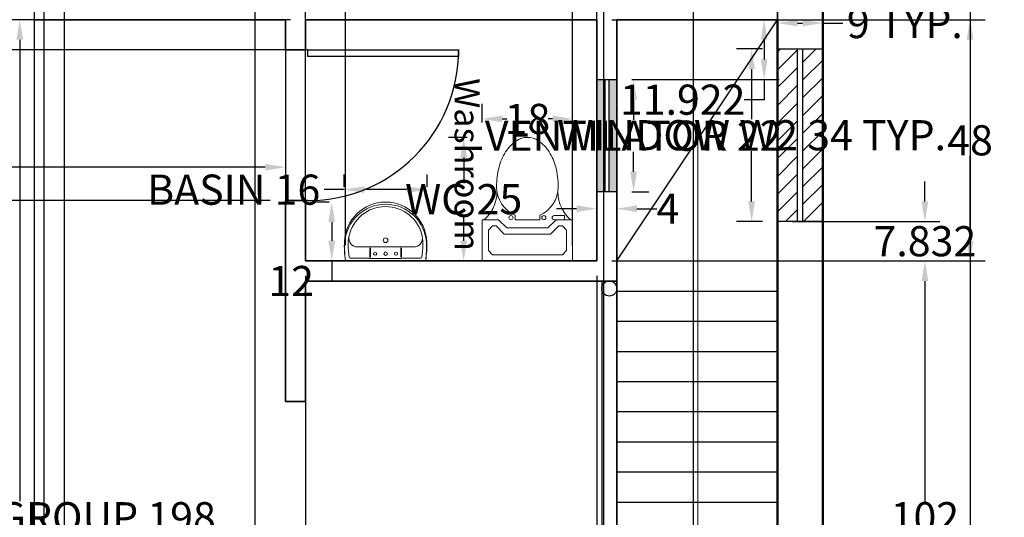
# Model space of a CAD drawing. Units: inches. Extents: x -1285 to -837, y -84 to 552.
# Tile 9 of 10: x -1037 to -841, y 263 to 362. Entities that reach past the tile are written whole.
import ezdxf

# ---------------------------------------------------------------- set-up
doc = ezdxf.new("R2010")
doc.units = ezdxf.units.IN
doc.header["$MEASUREMENT"] = 0
for name, color, linetype, lineweight in [('A-ANNO-DIMS', 2, 'Continuous', 18), ('A-ANNO-SYMB', 7, 'Continuous', 18), ('A-AREA-IDEN', 7, 'Continuous', 25), ('A-GLAZ-PATT', 191, 'Continuous', 13), ('A-GLAZ-VENT-PATT', 130, 'Continuous', 13), ('Commode', 60, 'Continuous', 18), ('Doors', 34, 'Continuous', 25), ('Inner Wall', 202, 'Continuous', 35), ('Outer Wall', 12, 'Continuous', 50), ('Sink', 33, 'Continuous', 18), ('Stairs', 90, 'Continuous', 25), ('Ventilators', 130, 'Continuous', 25), ('Windows', 191, 'Continuous', 25)]:
    doc.layers.add(name, color=color, linetype=linetype, lineweight=lineweight)
doc.styles.get("Standard").update_dxf_attribs({"font": 'arial.ttf'})
doc.dimstyles.get("Standard").update_dxf_attribs({"dimtxt": 6, "dimasz": 4, "dimexe": 3, "dimexo": 3, "dimgap": 0.09, "dimtad": 0, "dimtih": 1, "dimtoh": 1, "dimdec": 1, "dimzin": 0, "dimdsep": 46, "dimlunit": 3, "dimtxsty": 'Standard', "dimcen": 0.09, "dimadec": 0, "dimazin": 0, "dimtfac": 1, "dimtdec": 1, "dimtofl": 0, "dimtmove": 0, "dimatfit": 3, "dimfxl": 1, "dimtolj": 1, "dimtzin": 0, "dimarcsym": 0})

# ---------------------------------------------------------------- blocks, each defined once
blk = doc.blocks.new('A$C5EF6120A')
at = {"linetype": 'ByBlock'}
for p, q in [((0, 0.762), (0, 0.508)), ((0, 0.762), (0.5588, 0.762)), ((0.5588, 0.762), (0.5588, 0.508)), ((0.0381, 0.6985), (0.0635, 0.7239)), ((0.0381, 0.6985), (0.0381, 0.5715)), ((0.0635, 0.7239), (0.4953, 0.7239)), ((0.4953, 0.7239), (0.5207, 0.6985)), ((0.5207, 0.6985), (0.5207, 0.5715)), ((0.0635, 0.5461), (0.0381, 0.5715)), ((0.1366, 0.5969), (0.0858, 0.5461)), ((0.1524, 0.5588), (0.1016, 0.508)), ((0.1366, 0.5969), (0.4222, 0.5969)), ((0.1524, 0.5588), (0.4064, 0.5588)), ((0.4064, 0.5588), (0.4572, 0.508)), ((0.4222, 0.5969), (0.473, 0.5461)), ((0.5207, 0.5715), (0.4953, 0.5461)), ((0, 0.508), (0.1016, 0.508)), ((0.0508, 0.508), (0.0508, 0.4826)), ((0.0635, 0.5461), (0.0858, 0.5461)), ((0.1143, 0.508), (0.1016, 0.508)), ((0.2032, 0.508), (0.2032, 0.4794)), ((0.3556, 0.508), (0.2032, 0.508)), ((0.3556, 0.508), (0.3556, 0.4794)), ((0.5588, 0.508), (0.4572, 0.508)), ((0.4953, 0.5461), (0.473, 0.5461)), ((0.0508, 0.4826), (0.1143, 0.4826))]:
    blk.add_line(p, q, dxfattribs=at)
blk.add_lwpolyline([(0.0889, 0.3048, 0.063415), (0.1044, 0.183, 0.076468), (0.1447, 0.0893, 0.107136), (0.2118, 0.0204, 0.147373), (0.2794, 0, 0.147373), (0.347, 0.0204, 0.107136), (0.4141, 0.0893, 0.076468), (0.4544, 0.183, 0.063415), (0.4699, 0.3048, 0.063415)], format="xyb", dxfattribs=at)
for centre in [(0.1778, 0.4953), (0.381, 0.4953)]:
    blk.add_circle(centre, 0.0127, dxfattribs=at)
for centre, radius, start, end in [((-0.1375, 0.3358), 0.2285, 352.20108, 48.91101), ((0.1143, 0.4953), 0.0127, 270, 90), ((0.6963, 0.3358), 0.2285, 131.08899, 187.79892), ((0.2794, 0.3048), 0.1905, 113.57818, 180), ((0.2794, 0.3048), 0.1905, 0, 66.42182)]:
    blk.add_arc(centre, radius, start, end, dxfattribs=at)
blk = doc.blocks.new('B1')
at = {"color": 0}
for p, q in [((-342.1, -28), (-155.1, -28)), ((-153.6, -35.9), (-153.6, -126.6)), ((-147.1, -24), (-0.5, -24)), ((-147.1, -35.9), (-147.1, -126.6)), ((147.1, -24), (-0.5, -24)), ((147.1, -35.9), (147.1, -126.6)), ((153.6, -35.9), (153.6, -126.6)), ((342.1, -28), (155.1, -28)), ((-0.5, -135), (-272, -135)), ((-0.5, -135), (272.1, -135))]:
    blk.add_line(p, q, dxfattribs=at)
blk.add_lwpolyline([(0, -570, -0.403574), (-399.2, -186.1, -0.04955), (-388.9, -8.4, -0.368901), (-379, 0), (0, 0), (379.1, 0, -0.368901), (388.9, -8.4, -0.04955), (399.3, -186.1, -0.40261)], format="xyb", close=True, dxfattribs=at)
for centre in [(-100.5, -70), (100.6, -70)]:
    blk.add_circle(centre, 15, dxfattribs=at)
for centre, radius, start, end in [((502.9, -129.4), 900, 172.27277, 182.73185), ((437.5, -165.7), 800, 170.69697, 179.27367), ((-342.1, -38), 10, 90, 170.69697), ((-155.1, -24), 4, 270, 323.1301), ((-147.1, -30), 6, 90, 143.1301), ((-0.5, -70), 17.5, 90, 270), ((-0.5, -70), 17.5, 270, 90), ((147.1, -30), 6, 36.8699, 90), ((155.1, -24), 4, 216.8699, 270), ((342.1, -38), 10, 9.30303, 90), ((-437.5, -165.7), 800, 0.72633, 9.30303), ((-502.9, -129.4), 900, 357.26815, 7.72723), ((-0.5, -153), 396, 182.79964, 270.07706), ((-0.5, -165), 362, 178.50683, 191.45253), ((-272, -220), 85, 90, 191.45253), ((0, -200), 23, 90, 270), ((-0.4, -152), 397, 270.055, 357.0633), ((0, -200), 23, 270, 90), ((272.1, -220), 85, 348.54747, 90), ((0.6, -165), 362, 348.54747, 1.49317), ((-0.5, -165), 362, 191.45253, 270.0843), ((-0.4, -163.8), 363.2, 270.06445, 348.39326)]:
    blk.add_arc(centre, radius, start, end, dxfattribs=at)
blk = doc.blocks.new('*U17')
for p, q in [((-40, 0), (-40, 6)), ((0, 0), (0, 6))]:
    blk.add_line(p, q)
blk.add_lwpolyline([(0, 0), (0, -40), (-1.75, -40), (-1.75, 0)], close=True)
blk.add_arc((0, 0), 40, 180, 270)
blk = doc.blocks.new('Ventilator 1.1')
blk.add_line((1721.21, 1006.75), (1717.21, 1006.75))
at = {"layer": 'Ventilators'}
for p, q in [((1717.21, 1029.09), (1717.21, 1006.75)), ((1717.21, 1029.09), (1721.21, 1029.09)), ((1718.82, 1029.09), (1718.82, 1006.75)), ((1719.65, 1029.09), (1719.65, 1006.75)), ((1721.21, 1029.09), (1721.21, 1006.75))]:
    blk.add_line(p, q, dxfattribs=at)
blk = doc.blocks.new('WIN-34x9')
for p, q in [((4, 0), (4, 34.35)), ((5, 34.35), (5, 0))]:
    blk.add_line(p, q)
blk.add_lwpolyline([(9, 34.35), (9, 0), (0, 0), (0, 34.35)], close=True)
blk = doc.blocks.new('*D31')
at = {"layer": 'A-ANNO-DIMS', "color": 0, "lineweight": -2, "transparency": 16777216}
for p, q in [((-889.53, 356.12), (-894.68, 356.12)), ((-891.68, 352.12), (-891.68, 342.14)), ((-891.68, 325.77), (-891.68, 335.75)), ((-889.53, 321.77), (-894.68, 321.77))]:
    blk.add_line(p, q, dxfattribs=at)
at = {"layer": 'A-ANNO-DIMS', "color": 0, "transparency": 16777216}
for points in [[(-892.35, 352.12), (-891.02, 352.12), (-891.68, 356.12)], [(-892.35, 325.77), (-891.02, 325.77), (-891.68, 321.77)]]:
    blk.add_solid(points, dxfattribs=at)
at = {"layer": 'Defpoints', "color": 0, "transparency": 16777216}
for p in [(-891.68, 356.12), (-886.53, 356.12), (-886.53, 321.77)]:
    blk.add_point(p, dxfattribs=at)
at = {"layer": 'A-ANNO-DIMS', "color": 0, "transparency": 16777216, "insert": (-891.68, 338.95), "char_height": 6, "attachment_point": 5}
blk.add_mtext('\\A1;WINDOW W2 34 TYP.', dxfattribs=at)
blk = doc.blocks.new('*D32')
at = {"layer": 'A-ANNO-DIMS', "color": 0, "lineweight": -2, "transparency": 16777216}
for p, q in [((-886.53, 359.12), (-886.53, 364.27)), ((-877.53, 359.12), (-877.53, 364.27)), ((-882.53, 361.27), (-881.53, 361.27)), ((-877.53, 361.27), (-873.53, 361.27))]:
    blk.add_line(p, q, dxfattribs=at)
at = {"layer": 'A-ANNO-DIMS', "color": 0, "transparency": 16777216}
for points in [[(-882.53, 361.94), (-882.53, 360.61), (-886.53, 361.27)], [(-881.53, 361.94), (-881.53, 360.61), (-877.53, 361.27)]]:
    blk.add_solid(points, dxfattribs=at)
at = {"layer": 'Defpoints', "color": 0, "transparency": 16777216}
for p in [(-877.53, 361.27), (-886.53, 356.12), (-877.53, 356.12)]:
    blk.add_point(p, dxfattribs=at)
at = {"layer": 'A-ANNO-DIMS', "color": 0, "transparency": 16777216, "insert": (-861.17, 361.27), "char_height": 6, "attachment_point": 5}
blk.add_mtext('\\A1;9 TYP.', dxfattribs=at)
blk = doc.blocks.new('*D35')
at = {"layer": 'A-ANNO-DIMS', "color": 0, "lineweight": -2, "transparency": 16777216}
for p, q in [((-948.34, 338.51), (-952.02, 338.51)), ((-949.02, 334.51), (-949.02, 329.42)), ((-949.02, 317.94), (-949.02, 323.03)), ((-948.34, 313.94), (-952.02, 313.94))]:
    blk.add_line(p, q, dxfattribs=at)
at = {"layer": 'A-ANNO-DIMS', "color": 0, "transparency": 16777216}
for points in [[(-949.69, 334.51), (-948.35, 334.51), (-949.02, 338.51)], [(-949.69, 317.94), (-948.35, 317.94), (-949.02, 313.94)]]:
    blk.add_solid(points, dxfattribs=at)
at = {"layer": 'Defpoints', "color": 0, "transparency": 16777216}
for p in [(-945.34, 338.51), (-949.02, 313.94), (-945.34, 313.94)]:
    blk.add_point(p, dxfattribs=at)
at = {"layer": 'A-ANNO-DIMS', "color": 0, "transparency": 16777216, "insert": (-949.02, 326.22), "char_height": 6, "attachment_point": 5}
blk.add_mtext('\\A1;WC 25', dxfattribs=at)
blk = doc.blocks.new('*D36')
at = {"layer": 'A-ANNO-DIMS', "color": 0, "lineweight": -2, "transparency": 16777216}
for p, q in [((-945.34, 341.51), (-945.34, 345.19)), ((-927.32, 341.51), (-927.32, 345.19)), ((-941.34, 342.19), (-940.44, 342.19)), ((-931.32, 342.19), (-932.22, 342.19))]:
    blk.add_line(p, q, dxfattribs=at)
at = {"layer": 'A-ANNO-DIMS', "color": 0, "transparency": 16777216}
for points in [[(-941.34, 342.86), (-941.34, 341.53), (-945.34, 342.19)], [(-931.32, 342.86), (-931.32, 341.53), (-927.32, 342.19)]]:
    blk.add_solid(points, dxfattribs=at)
at = {"layer": 'Defpoints', "color": 0, "transparency": 16777216}
for p in [(-945.34, 342.19), (-945.34, 338.51), (-927.32, 338.51)]:
    blk.add_point(p, dxfattribs=at)
at = {"layer": 'A-ANNO-DIMS', "color": 0, "transparency": 16777216, "insert": (-936.33, 342.19), "char_height": 6, "attachment_point": 5}
blk.add_mtext('\\A1;18', dxfattribs=at)
blk = doc.blocks.new('*D39')
at = {"layer": 'A-ANNO-DIMS', "color": 0, "lineweight": -2, "transparency": 16777216}
for p, q in [((-972.82, 328.65), (-972.82, 331.12)), ((-956.32, 328.65), (-956.32, 331.12)), ((-972.82, 328.12), (-976.82, 328.12)), ((-960.32, 328.12), (-968.82, 328.12))]:
    blk.add_line(p, q, dxfattribs=at)
at = {"layer": 'A-ANNO-DIMS', "color": 0, "transparency": 16777216}
for points in [[(-968.82, 328.79), (-968.82, 327.46), (-972.82, 328.12)], [(-960.32, 328.79), (-960.32, 327.46), (-956.32, 328.12)]]:
    blk.add_solid(points, dxfattribs=at)
at = {"layer": 'Defpoints', "color": 0, "transparency": 16777216}
for p in [(-972.82, 328.12), (-972.82, 325.65), (-956.32, 325.65)]:
    blk.add_point(p, dxfattribs=at)
at = {"layer": 'A-ANNO-DIMS', "color": 0, "transparency": 16777216, "insert": (-994.81, 328.12), "char_height": 6, "attachment_point": 5}
blk.add_mtext('\\A1;BASIN 16', dxfattribs=at)
blk = doc.blocks.new('*D40')
at = {"layer": 'A-ANNO-DIMS', "color": 0, "lineweight": -2, "transparency": 16777216}
for p, q in [((-975.82, 325.65), (-978.29, 325.65)), ((-975.29, 321.65), (-975.29, 317.94)), ((-975.82, 313.94), (-978.29, 313.94)), ((-975.29, 313.94), (-975.29, 309.94)), ((-975.29, 309.94), (-979.29, 309.94))]:
    blk.add_line(p, q, dxfattribs=at)
at = {"layer": 'A-ANNO-DIMS', "color": 0, "transparency": 16777216}
for points in [[(-975.96, 321.65), (-974.63, 321.65), (-975.29, 325.65)], [(-975.96, 317.94), (-974.63, 317.94), (-975.29, 313.94)]]:
    blk.add_solid(points, dxfattribs=at)
at = {"layer": 'Defpoints', "color": 0, "transparency": 16777216}
for p in [(-972.82, 325.65), (-975.29, 313.94), (-972.82, 313.94)]:
    blk.add_point(p, dxfattribs=at)
at = {"layer": 'A-ANNO-DIMS', "color": 0, "transparency": 16777216, "insert": (-983.37, 309.94), "char_height": 6, "attachment_point": 5}
blk.add_mtext('\\A1;12', dxfattribs=at)
blk = doc.blocks.new('*D65')
at = {"layer": 'A-ANNO-DIMS', "color": 0, "lineweight": -2, "transparency": 16777216}
for p, q in [((-1064.13, 361.96), (-1034.42, 361.96)), ((-1037.42, 357.96), (-1037.42, 266.12)), ((-1037.42, 167.9), (-1037.42, 259.73)), ((-1064.13, 163.9), (-1034.42, 163.9))]:
    blk.add_line(p, q, dxfattribs=at)
at = {"layer": 'A-ANNO-DIMS', "color": 0, "transparency": 16777216}
for points in [[(-1038.09, 357.96), (-1036.75, 357.96), (-1037.42, 361.96)], [(-1038.09, 167.9), (-1036.75, 167.9), (-1037.42, 163.9)]]:
    blk.add_solid(points, dxfattribs=at)
at = {"layer": 'Defpoints', "color": 0, "transparency": 16777216}
for p in [(-1067.13, 361.96), (-1037.42, 361.96), (-1067.13, 163.9)]:
    blk.add_point(p, dxfattribs=at)
at = {"layer": 'A-ANNO-DIMS', "color": 0, "transparency": 16777216, "insert": (-1037.42, 262.93), "char_height": 6, "attachment_point": 5}
blk.add_mtext('\\A1;LOUNGE GROUP 198', dxfattribs=at)
blk = doc.blocks.new('*D67')
at = {"layer": 'A-ANNO-DIMS', "color": 0, "lineweight": -2, "transparency": 16777216}
for p, q in [((-915.53, 350.02), (-912.18, 350.02)), ((-915.18, 346.02), (-915.18, 342.04)), ((-915.18, 331.68), (-915.18, 335.65)), ((-915.53, 327.68), (-912.18, 327.68))]:
    blk.add_line(p, q, dxfattribs=at)
at = {"layer": 'A-ANNO-DIMS', "color": 0, "transparency": 16777216}
for points in [[(-915.85, 346.02), (-914.51, 346.02), (-915.18, 350.02)], [(-915.85, 331.68), (-914.51, 331.68), (-915.18, 327.68)]]:
    blk.add_solid(points, dxfattribs=at)
at = {"layer": 'Defpoints', "color": 0, "transparency": 16777216}
for p in [(-918.53, 350.02), (-915.18, 350.02), (-918.53, 327.68)]:
    blk.add_point(p, dxfattribs=at)
at = {"layer": 'A-ANNO-DIMS', "color": 0, "transparency": 16777216, "insert": (-915.18, 338.85), "char_height": 6, "attachment_point": 5}
blk.add_mtext('\\A1;VENTILATOR 22', dxfattribs=at)
blk = doc.blocks.new('*D68')
at = {"layer": 'A-ANNO-DIMS', "color": 0, "lineweight": -2, "transparency": 16777216}
for p, q in [((-926.53, 324.33), (-930.53, 324.33)), ((-922.53, 324.68), (-922.53, 321.33)), ((-918.53, 324.68), (-918.53, 321.33)), ((-914.53, 324.33), (-910.53, 324.33))]:
    blk.add_line(p, q, dxfattribs=at)
at = {"layer": 'A-ANNO-DIMS', "color": 0, "transparency": 16777216}
for points in [[(-926.53, 325), (-926.53, 323.66), (-922.53, 324.33)], [(-914.53, 325), (-914.53, 323.66), (-918.53, 324.33)]]:
    blk.add_solid(points, dxfattribs=at)
at = {"layer": 'Defpoints', "color": 0, "transparency": 16777216}
for p in [(-922.53, 327.68), (-918.53, 327.68), (-918.53, 324.33)]:
    blk.add_point(p, dxfattribs=at)
at = {"layer": 'A-ANNO-DIMS', "color": 0, "transparency": 16777216, "insert": (-908.36, 324.33), "char_height": 6, "attachment_point": 5}
blk.add_mtext('\\A1;4', dxfattribs=at)
blk = doc.blocks.new('*D70')
at = {"layer": 'A-ANNO-DIMS', "color": 0, "lineweight": -2, "transparency": 16777216}
for p, q in [((-874.53, 518.94), (-845.18, 518.94)), ((-848.18, 514.94), (-848.18, 237.09)), ((-848.18, -47.06), (-848.18, 230.79)), ((-874.53, -51.06), (-845.18, -51.06))]:
    blk.add_line(p, q, dxfattribs=at)
at = {"layer": 'A-ANNO-DIMS', "color": 0, "transparency": 16777216}
for points in [[(-848.85, 514.94), (-847.51, 514.94), (-848.18, 518.94)], [(-848.85, -47.06), (-847.51, -47.06), (-848.18, -51.06)]]:
    blk.add_solid(points, dxfattribs=at)
at = {"layer": 'Defpoints', "color": 0, "transparency": 16777216}
for p in [(-877.53, 518.94), (-848.18, 518.94), (-877.53, -51.06)]:
    blk.add_point(p, dxfattribs=at)
at = {"layer": 'A-ANNO-DIMS', "color": 0, "transparency": 16777216, "insert": (-848.18, 233.94), "char_height": 6, "attachment_point": 5}
blk.add_mtext('\\A1;570', dxfattribs=at)
blk = doc.blocks.new('*D80')
at = {"layer": 'A-ANNO-DIMS', "color": 0, "lineweight": -2, "transparency": 16777216}
for p, q in [((-1184.53, -13.66), (-1184.53, 551.29)), ((-1032.53, -13.66), (-1032.53, 551.29)), ((-1180.53, 548.29), (-1114.94, 548.29)), ((-1036.53, 548.29), (-1102.12, 548.29))]:
    blk.add_line(p, q, dxfattribs=at)
at = {"layer": 'A-ANNO-DIMS', "color": 0, "transparency": 16777216}
for points in [[(-1180.53, 548.96), (-1180.53, 547.62), (-1184.53, 548.29)], [(-1036.53, 548.96), (-1036.53, 547.62), (-1032.53, 548.29)]]:
    blk.add_solid(points, dxfattribs=at)
at = {"layer": 'Defpoints', "color": 0, "transparency": 16777216}
for p in [(-1032.53, 548.29), (-1184.53, -16.66), (-1032.53, -16.66)]:
    blk.add_point(p, dxfattribs=at)
at = {"layer": 'A-ANNO-DIMS', "color": 0, "transparency": 16777216, "insert": (-1108.53, 548.29), "char_height": 6, "attachment_point": 5}
blk.add_mtext('\\A1;152', dxfattribs=at)
blk = doc.blocks.new('*D84')
at = {"layer": 'A-ANNO-DIMS', "color": 0, "lineweight": -2, "transparency": 16777216}
for p, q in [((-919.53, 361.94), (-845.18, 361.94)), ((-848.18, 357.94), (-848.18, 341.09)), ((-848.18, 317.94), (-848.18, 334.79)), ((-919.53, 313.94), (-845.18, 313.94))]:
    blk.add_line(p, q, dxfattribs=at)
at = {"layer": 'A-ANNO-DIMS', "color": 0, "transparency": 16777216}
for points in [[(-848.85, 357.94), (-847.51, 357.94), (-848.18, 361.94)], [(-848.85, 317.94), (-847.51, 317.94), (-848.18, 313.94)]]:
    blk.add_solid(points, dxfattribs=at)
at = {"layer": 'Defpoints', "color": 0, "transparency": 16777216}
for p in [(-922.53, 361.94), (-848.18, 361.94), (-922.53, 313.94)]:
    blk.add_point(p, dxfattribs=at)
at = {"layer": 'A-ANNO-DIMS', "color": 0, "transparency": 16777216, "insert": (-848.18, 337.94), "char_height": 6, "attachment_point": 5}
blk.add_mtext('\\A1;48', dxfattribs=at)
blk = doc.blocks.new('*D85')
at = {"layer": 'A-ANNO-DIMS', "color": 0, "lineweight": -2, "transparency": 16777216}
for p, q in [((-980.53, 310.94), (-980.53, -83.53)), ((-922.53, 310.94), (-922.53, -83.53)), ((-976.53, -80.53), (-955.92, -80.53)), ((-926.53, -80.53), (-947.14, -80.53))]:
    blk.add_line(p, q, dxfattribs=at)
at = {"layer": 'A-ANNO-DIMS', "color": 0, "transparency": 16777216}
for points in [[(-976.53, -79.86), (-976.53, -81.2), (-980.53, -80.53)], [(-926.53, -79.86), (-926.53, -81.2), (-922.53, -80.53)]]:
    blk.add_solid(points, dxfattribs=at)
at = {"layer": 'Defpoints', "color": 0, "transparency": 16777216}
for p in [(-980.53, 313.94), (-922.53, 313.94), (-922.53, -80.53)]:
    blk.add_point(p, dxfattribs=at)
at = {"layer": 'A-ANNO-DIMS', "color": 0, "transparency": 16777216, "insert": (-951.53, -80.53), "char_height": 6, "attachment_point": 5}
blk.add_mtext('\\A1;58', dxfattribs=at)
blk = doc.blocks.new('*D86')
at = {"layer": 'A-ANNO-DIMS', "color": 0, "lineweight": -2, "transparency": 16777216}
for p, q in [((-918.53, 310.94), (-918.53, -83.53)), ((-886.53, 310.94), (-886.53, -83.53)), ((-914.53, -80.53), (-906.88, -80.53)), ((-890.53, -80.53), (-898.18, -80.53))]:
    blk.add_line(p, q, dxfattribs=at)
at = {"layer": 'A-ANNO-DIMS', "color": 0, "transparency": 16777216}
for points in [[(-914.53, -79.86), (-914.53, -81.2), (-918.53, -80.53)], [(-890.53, -79.86), (-890.53, -81.2), (-886.53, -80.53)]]:
    blk.add_solid(points, dxfattribs=at)
at = {"layer": 'Defpoints', "color": 0, "transparency": 16777216}
for p in [(-918.53, 313.94), (-886.53, 313.94), (-886.53, -80.53)]:
    blk.add_point(p, dxfattribs=at)
at = {"layer": 'A-ANNO-DIMS', "color": 0, "transparency": 16777216, "insert": (-902.53, -80.53), "char_height": 6, "attachment_point": 5}
blk.add_mtext('\\A1;32', dxfattribs=at)
blk = doc.blocks.new('*D88')
at = {"layer": 'A-ANNO-DIMS', "color": 0, "lineweight": -2, "transparency": 16777216}
for p, q in [((-987.53, 355.94), (-1277.88, 355.94)), ((-1274.88, 351.94), (-1274.88, 344.09)), ((-1274.88, 329.94), (-1274.88, 337.78)), ((-987.53, 325.94), (-1277.88, 325.94))]:
    blk.add_line(p, q, dxfattribs=at)
at = {"layer": 'A-ANNO-DIMS', "color": 0, "transparency": 16777216}
for points in [[(-1275.55, 351.94), (-1274.21, 351.94), (-1274.88, 355.94)], [(-1275.55, 329.94), (-1274.21, 329.94), (-1274.88, 325.94)]]:
    blk.add_solid(points, dxfattribs=at)
at = {"layer": 'Defpoints', "color": 0, "transparency": 16777216}
for p in [(-1274.88, 355.94), (-984.53, 355.94), (-984.53, 325.94)]:
    blk.add_point(p, dxfattribs=at)
at = {"layer": 'A-ANNO-DIMS', "color": 0, "transparency": 16777216, "insert": (-1274.88, 340.94), "char_height": 6, "attachment_point": 5}
blk.add_mtext('\\A1;30', dxfattribs=at)
blk = doc.blocks.new('*D93')
at = {"layer": 'A-ANNO-DIMS', "color": 0, "lineweight": -2, "transparency": 16777216}
for p, q in [((-1028.53, 78.94), (-1028.53, 551.29)), ((-990.53, 78.94), (-990.53, 551.29)), ((-1024.53, 548.29), (-1013.92, 548.29)), ((-994.53, 548.29), (-1005.14, 548.29))]:
    blk.add_line(p, q, dxfattribs=at)
at = {"layer": 'A-ANNO-DIMS', "color": 0, "transparency": 16777216}
for points in [[(-1024.53, 548.96), (-1024.53, 547.62), (-1028.53, 548.29)], [(-994.53, 548.96), (-994.53, 547.62), (-990.53, 548.29)]]:
    blk.add_solid(points, dxfattribs=at)
at = {"layer": 'Defpoints', "color": 0, "transparency": 16777216}
for p in [(-990.53, 548.29), (-1028.53, 75.94), (-990.53, 75.94)]:
    blk.add_point(p, dxfattribs=at)
at = {"layer": 'A-ANNO-DIMS', "color": 0, "transparency": 16777216, "insert": (-1009.53, 548.29), "char_height": 6, "attachment_point": 5}
blk.add_mtext('\\A1;38', dxfattribs=at)
blk = doc.blocks.new('*D95')
at = {"layer": 'A-ANNO-DIMS', "color": 0, "lineweight": -2, "transparency": 16777216}
for p, q in [((-883.53, 313.94), (-854.18, 313.94)), ((-857.18, 309.94), (-857.18, 266.09)), ((-857.18, 215.94), (-857.18, 259.79)), ((-883.53, 211.94), (-854.18, 211.94))]:
    blk.add_line(p, q, dxfattribs=at)
at = {"layer": 'A-ANNO-DIMS', "color": 0, "transparency": 16777216}
for points in [[(-857.85, 309.94), (-856.51, 309.94), (-857.18, 313.94)], [(-857.85, 215.94), (-856.51, 215.94), (-857.18, 211.94)]]:
    blk.add_solid(points, dxfattribs=at)
at = {"layer": 'Defpoints', "color": 0, "transparency": 16777216}
for p in [(-886.53, 313.94), (-886.53, 211.94), (-857.18, 211.94)]:
    blk.add_point(p, dxfattribs=at)
at = {"layer": 'A-ANNO-DIMS', "color": 0, "transparency": 16777216, "insert": (-857.18, 262.94), "char_height": 6, "attachment_point": 5}
blk.add_mtext('\\A1;102', dxfattribs=at)
blk = doc.blocks.new('*D97')
at = {"layer": 'A-ANNO-DIMS', "color": 0, "lineweight": -2, "transparency": 16777216}
for p, q in [((-921.19, 506.94), (-921.19, -83.53)), ((-886.53, 506.94), (-886.53, -83.53)), ((-917.19, -80.53), (-916.43, -80.53)), ((-890.53, -80.53), (-891.3, -80.53))]:
    blk.add_line(p, q, dxfattribs=at)
at = {"layer": 'A-ANNO-DIMS', "color": 0, "transparency": 16777216}
for points in [[(-917.19, -79.86), (-917.19, -81.2), (-921.19, -80.53)], [(-890.53, -79.86), (-890.53, -81.2), (-886.53, -80.53)]]:
    blk.add_solid(points, dxfattribs=at)
at = {"layer": 'Defpoints', "color": 0, "transparency": 16777216}
for p in [(-921.19, 509.94), (-886.53, 509.94), (-886.53, -80.53)]:
    blk.add_point(p, dxfattribs=at)
at = {"layer": 'A-ANNO-DIMS', "color": 0, "transparency": 16777216, "insert": (-903.86, -80.53), "char_height": 6, "attachment_point": 5}
blk.add_mtext('\\A1;34.665', dxfattribs=at)
blk = doc.blocks.new('*D102')
at = {"layer": 'A-ANNO-DIMS', "color": 0, "lineweight": -2, "transparency": 16777216}
for p, q in [((-903.24, -39.06), (-903.24, 551.29)), ((-886.53, -39.06), (-886.53, 551.29)), ((-899.24, 548.29), (-890.53, 548.29)), ((-886.53, 548.29), (-882.53, 548.29))]:
    blk.add_line(p, q, dxfattribs=at)
at = {"layer": 'A-ANNO-DIMS', "color": 0, "transparency": 16777216}
for points in [[(-899.24, 548.96), (-899.24, 547.62), (-903.24, 548.29)], [(-890.53, 548.96), (-890.53, 547.62), (-886.53, 548.29)]]:
    blk.add_solid(points, dxfattribs=at)
at = {"layer": 'Defpoints', "color": 0, "transparency": 16777216}
for p in [(-886.53, 548.29), (-903.24, -42.06), (-886.53, -42.06)]:
    blk.add_point(p, dxfattribs=at)
at = {"layer": 'A-ANNO-DIMS', "color": 0, "transparency": 16777216, "insert": (-873.18, 548.29), "char_height": 6, "attachment_point": 5}
blk.add_mtext('\\A1;16.71', dxfattribs=at)
blk = doc.blocks.new('*D104')
at = {"layer": 'A-ANNO-DIMS', "color": 0, "lineweight": -2, "transparency": 16777216}
for p, q in [((-1044.37, 506.94), (-1044.37, -83.53)), ((-1034.53, 506.94), (-1034.53, -83.53)), ((-1040.37, -80.53), (-1038.53, -80.53)), ((-1034.53, -80.53), (-1030.53, -80.53))]:
    blk.add_line(p, q, dxfattribs=at)
at = {"layer": 'A-ANNO-DIMS', "color": 0, "transparency": 16777216}
for points in [[(-1040.37, -79.86), (-1040.37, -81.2), (-1044.37, -80.53)], [(-1038.53, -79.86), (-1038.53, -81.2), (-1034.53, -80.53)]]:
    blk.add_solid(points, dxfattribs=at)
at = {"layer": 'Defpoints', "color": 0, "transparency": 16777216}
for p in [(-1044.37, 509.94), (-1034.53, 509.94), (-1034.53, -80.53)]:
    blk.add_point(p, dxfattribs=at)
at = {"layer": 'A-ANNO-DIMS', "color": 0, "transparency": 16777216, "insert": (-1022.66, -80.53), "char_height": 6, "attachment_point": 5}
blk.add_mtext('\\A1;9.84', dxfattribs=at)
blk = doc.blocks.new('*D106')
at = {"layer": 'A-ANNO-DIMS', "color": 0, "lineweight": -2, "transparency": 16777216}
for p, q in [((-1274.88, 365.94), (-1274.88, 369.94)), ((-1274.88, 369.94), (-1270.88, 369.94)), ((-983.53, 361.94), (-1277.88, 361.94)), ((-983.53, 355.94), (-1277.88, 355.94)), ((-1274.88, 351.94), (-1274.88, 347.94))]:
    blk.add_line(p, q, dxfattribs=at)
at = {"layer": 'A-ANNO-DIMS', "color": 0, "transparency": 16777216}
for points in [[(-1275.55, 365.94), (-1274.21, 365.94), (-1274.88, 361.94)], [(-1275.55, 351.94), (-1274.21, 351.94), (-1274.88, 355.94)]]:
    blk.add_solid(points, dxfattribs=at)
at = {"layer": 'Defpoints', "color": 0, "transparency": 16777216}
for p in [(-1274.88, 361.94), (-980.53, 361.94), (-980.53, 355.94)]:
    blk.add_point(p, dxfattribs=at)
at = {"layer": 'A-ANNO-DIMS', "color": 0, "transparency": 16777216, "insert": (-1268.81, 369.94), "char_height": 6, "attachment_point": 5}
blk.add_mtext('\\A1;6', dxfattribs=at)
blk = doc.blocks.new('*D107')
at = {"layer": 'A-ANNO-DIMS', "color": 0, "lineweight": -2, "transparency": 16777216}
for p, q in [((-980.53, 316.94), (-980.53, 551.29)), ((-972.53, 317.04), (-972.53, 551.29)), ((-984.53, 548.29), (-988.53, 548.29)), ((-968.53, 548.29), (-964.53, 548.29))]:
    blk.add_line(p, q, dxfattribs=at)
at = {"layer": 'A-ANNO-DIMS', "color": 0, "transparency": 16777216}
for points in [[(-984.53, 548.96), (-984.53, 547.62), (-980.53, 548.29)], [(-968.53, 548.96), (-968.53, 547.62), (-972.53, 548.29)]]:
    blk.add_solid(points, dxfattribs=at)
at = {"layer": 'Defpoints', "color": 0, "transparency": 16777216}
for p in [(-972.53, 548.29), (-980.53, 313.94), (-972.53, 314.04)]:
    blk.add_point(p, dxfattribs=at)
at = {"layer": 'A-ANNO-DIMS', "color": 0, "transparency": 16777216, "insert": (-954.34, 548.29), "char_height": 6, "attachment_point": 5}
blk.add_mtext('\\A1;7.997', dxfattribs=at)
blk = doc.blocks.new('*D108')
at = {"layer": 'A-ANNO-DIMS', "color": 0, "lineweight": -2, "transparency": 16777216}
for p, q in [((-927.32, 316.94), (-927.32, 551.29)), ((-922.53, 316.94), (-922.53, 551.29)), ((-931.32, 548.29), (-935.32, 548.29)), ((-918.53, 548.29), (-914.53, 548.29))]:
    blk.add_line(p, q, dxfattribs=at)
at = {"layer": 'A-ANNO-DIMS', "color": 0, "transparency": 16777216}
for points in [[(-931.32, 548.96), (-931.32, 547.62), (-927.32, 548.29)], [(-918.53, 548.96), (-918.53, 547.62), (-922.53, 548.29)]]:
    blk.add_solid(points, dxfattribs=at)
at = {"layer": 'Defpoints', "color": 0, "transparency": 16777216}
for p in [(-922.53, 548.29), (-927.32, 313.94), (-922.53, 313.94)]:
    blk.add_point(p, dxfattribs=at)
at = {"layer": 'A-ANNO-DIMS', "color": 0, "transparency": 16777216, "insert": (-904.19, 548.29), "char_height": 6, "attachment_point": 5}
blk.add_mtext('\\A1;4.788', dxfattribs=at)
blk = doc.blocks.new('*D116')
at = {"layer": 'A-ANNO-DIMS', "color": 0, "lineweight": -2, "transparency": 16777216}
for p, q in [((-857.18, 325.77), (-857.18, 329.77)), ((-883.53, 321.77), (-854.18, 321.77)), ((-883.53, 313.94), (-854.18, 313.94)), ((-857.18, 309.94), (-857.18, 305.94))]:
    blk.add_line(p, q, dxfattribs=at)
at = {"layer": 'A-ANNO-DIMS', "color": 0, "transparency": 16777216}
for points in [[(-857.85, 325.77), (-856.51, 325.77), (-857.18, 321.77)], [(-857.85, 309.94), (-856.51, 309.94), (-857.18, 313.94)]]:
    blk.add_solid(points, dxfattribs=at)
at = {"layer": 'Defpoints', "color": 0, "transparency": 16777216}
for p in [(-886.53, 321.77), (-886.53, 313.94), (-857.18, 313.94)]:
    blk.add_point(p, dxfattribs=at)
at = {"layer": 'A-ANNO-DIMS', "color": 0, "transparency": 16777216, "insert": (-857.18, 317.86), "char_height": 6, "attachment_point": 5}
blk.add_mtext('\\A1;7.832', dxfattribs=at)
blk = doc.blocks.new('*D117')
at = {"layer": 'A-ANNO-DIMS', "color": 0, "lineweight": -2, "transparency": 16777216}
for p, q in [((-915.53, 361.94), (-886.18, 361.94)), ((-889.18, 357.94), (-889.18, 354.02)), ((-915.53, 350.02), (-886.18, 350.02)), ((-889.18, 350.02), (-889.18, 346.02)), ((-889.18, 346.02), (-893.18, 346.02))]:
    blk.add_line(p, q, dxfattribs=at)
at = {"layer": 'A-ANNO-DIMS', "color": 0, "transparency": 16777216}
for points in [[(-889.85, 357.94), (-888.51, 357.94), (-889.18, 361.94)], [(-889.85, 354.02), (-888.51, 354.02), (-889.18, 350.02)]]:
    blk.add_solid(points, dxfattribs=at)
at = {"layer": 'Defpoints', "color": 0, "transparency": 16777216}
for p in [(-918.53, 361.94), (-918.53, 350.02), (-889.18, 350.02)]:
    blk.add_point(p, dxfattribs=at)
at = {"layer": 'A-ANNO-DIMS', "color": 0, "transparency": 16777216, "insert": (-905.41, 346.02), "char_height": 6, "attachment_point": 5}
blk.add_mtext('\\A1;11.922', dxfattribs=at)
blk = doc.blocks.new('*D119')
at = {"layer": 'A-ANNO-DIMS', "color": 0, "lineweight": -2, "transparency": 16777216}
for p, q in [((-1236.53, 358.94), (-1236.53, 329.59)), ((-984.53, 358.94), (-984.53, 329.59)), ((-1232.53, 332.59), (-1117.27, 332.59)), ((-988.53, 332.59), (-1103.79, 332.59))]:
    blk.add_line(p, q, dxfattribs=at)
at = {"layer": 'A-ANNO-DIMS', "color": 0, "transparency": 16777216}
for points in [[(-1232.53, 333.26), (-1232.53, 331.92), (-1236.53, 332.59)], [(-988.53, 333.26), (-988.53, 331.92), (-984.53, 332.59)]]:
    blk.add_solid(points, dxfattribs=at)
at = {"layer": 'Defpoints', "color": 0, "transparency": 16777216}
for p in [(-1236.53, 361.94), (-984.53, 361.94), (-1236.53, 332.59)]:
    blk.add_point(p, dxfattribs=at)
at = {"layer": 'A-ANNO-DIMS', "color": 0, "transparency": 16777216, "insert": (-1110.53, 332.59), "char_height": 6, "attachment_point": 5}
blk.add_mtext('\\A1;252', dxfattribs=at)

msp = doc.modelspace()

# ---------------------------------------------------------------- hatches: boundary and pattern name
at = {"layer": 'A-GLAZ-PATT'}
h = msp.add_hatch(dxfattribs=at)
h.set_pattern_fill('ANSI31', color=256, scale=20)
h.set_pattern_definition([(45, (-2191.666, -702.1458), (-1.767767, 1.767767), [])])
h.paths.add_polyline_path([(-921.1945, 518.9392), (-984.2307, 518.9392), (-984.2307, 514.9392), (-921.1945, 514.9392)])
h.paths.add_polyline_path([(-921.1945, 513.9392), (-984.2307, 513.9392), (-984.2307, 509.9392), (-921.1945, 509.9392)])
h.paths.add_polyline_path([(-877.5299, 480.0491), (-881.5299, 480.0491), (-881.5299, 417.0129), (-877.5299, 417.0129)])
h.paths.add_polyline_path([(-882.5299, 480.0491), (-886.5299, 480.0491), (-886.5299, 417.0129), (-882.5299, 417.0129)])
h.paths.add_polyline_path([(-877.5299, 356.1195), (-881.5299, 356.1195), (-881.5299, 321.7709), (-877.5299, 321.7709)])
h.paths.add_polyline_path([(-882.5299, 356.1195), (-886.5299, 356.1195), (-886.5299, 321.7709), (-882.5299, 321.7709)])
h.paths.add_polyline_path([(-1133.8033, 518.9392), (-1196.8396, 518.9392), (-1196.8396, 514.9392), (-1133.8033, 514.9392)])
h.paths.add_polyline_path([(-1133.8033, 513.9392), (-1196.8396, 513.9392), (-1196.8396, 509.9392), (-1133.8033, 509.9392)])
h.paths.add_polyline_path([(-1236.5299, 138.1751), (-1240.5299, 138.1751), (-1240.5299, 75.1388), (-1236.5299, 75.1388)])
h.paths.add_polyline_path([(-1241.5299, 138.1751), (-1245.5299, 138.1751), (-1245.5299, 75.1388), (-1241.5299, 75.1388)])
h.paths.add_polyline_path([(-1236.5299, 35.9392), (-1240.5299, 35.9392), (-1240.5299, 1.5906), (-1236.5299, 1.5906)])
h.paths.add_polyline_path([(-1241.5299, 35.9392), (-1245.5299, 35.9392), (-1245.5299, 1.5906), (-1241.5299, 1.5906)])
h.paths.add_polyline_path([(-1088.8155, -16.6608), (-1136.8155, -16.6608), (-1136.8155, -20.6608), (-1088.8155, -20.6608)])
h.paths.add_polyline_path([(-1088.8155, -21.6608), (-1136.8155, -21.6608), (-1136.8155, -25.6608), (-1088.8155, -25.6608)])
at = {"layer": 'A-GLAZ-VENT-PATT'}
h = msp.add_hatch(color=256, dxfattribs=at)
h.dxf.hatch_style = 1
h.paths.add_polyline_path([(-920.9171, 350.017), (-922.5299, 350.017), (-922.5299, 327.6809), (-920.9171, 327.6809)])
h.paths.add_polyline_path([(-918.5299, 350.017), (-920.0891, 350.017), (-920.0891, 327.6809), (-918.5299, 327.6809)])

# ---------------------------------------------------------------- linework, layer by layer
at = {"layer": 'A-ANNO-SYMB'}
msp.add_line((-902.4002, 338.1338), (-902.4002, 185.376), dxfattribs=at)
at = {"layer": 'Inner Wall'}
for p, q in [((-1034.5299, 361.9392), (-984.5299, 361.9392)), ((-984.5299, 361.9392), (-984.5299, 355.9392)), ((-980.5299, 361.9392), (-980.5299, 355.9392)), ((-980.5299, 361.9392), (-922.5299, 361.9392)), ((-922.5299, 361.9392), (-922.5299, 313.9392)), ((-918.5299, 361.9392), (-918.5299, 211.9392)), ((-918.5299, 361.9392), (-886.5299, 361.9392)), ((-984.5299, 355.9392), (-980.5299, 355.9392)), ((-984.5299, 325.9392), (-980.5299, 325.9392)), ((-984.5299, 325.9392), (-984.5299, 285.9392)), ((-980.5299, 325.9392), (-980.5299, 313.9392)), ((-980.5299, 313.9392), (-922.5299, 313.9392)), ((-980.5299, 309.9392), (-918.5299, 309.9392)), ((-980.5299, 309.9392), (-980.5299, 285.9392)), ((-984.5299, 285.9392), (-980.5299, 285.9392))]:
    msp.add_line(p, q, dxfattribs=at)
at = {"layer": 'Outer Wall'}
for p, q in [((-877.5299, 518.9392), (-877.5299, -51.0608)), ((-886.5299, 361.9392), (-886.5299, 163.9392))]:
    msp.add_line(p, q, dxfattribs=at)
at = {"layer": 'Stairs'}
for p, q in [((-918.5299, 313.9392), (-886.5299, 361.9392)), ((-918.5299, 313.9392), (-886.5299, 313.9392)), ((-921.5299, 309.9392), (-921.5299, 214.9392)), ((-918.5299, 307.9392), (-886.5299, 307.9392)), ((-918.5299, 301.9392), (-886.5299, 301.9392)), ((-918.5299, 295.9392), (-886.5299, 295.9392)), ((-918.5299, 289.9392), (-886.5299, 289.9392)), ((-918.5299, 283.9392), (-886.5299, 283.9392)), ((-918.5299, 277.9392), (-886.5299, 277.9392)), ((-918.5299, 271.9392), (-886.5299, 271.9392)), ((-918.5299, 265.9392), (-886.5299, 265.9392))]:
    msp.add_line(p, q, dxfattribs=at)
msp.add_circle((-920.0299, 308.4392), 1.5, dxfattribs=at)

# ---------------------------------------------------------------- block references
at = {"layer": 'Commode', "xscale": 32.24256021731278, "yscale": 32.24256021731278, "zscale": 32.24256021731278, "rotation": 180}
msp.add_blockref('A$C5EF6120A', (-927.318, 338.5081), dxfattribs=at)
at = {"layer": 'Doors', "xscale": 0.75, "yscale": 0.75, "zscale": 0.75, "rotation": 90}
msp.add_blockref('*U17', (-980.0299, 355.9392), dxfattribs=at)
at = {"layer": 'Sink', "xscale": 0.0205351379380838, "yscale": 0.0205351379380838, "zscale": 0.0205351379380838, "rotation": 180}
msp.add_blockref('B1', (-964.5702, 313.9392), dxfattribs=at)
at = {"layer": 'Ventilators'}
msp.add_blockref('Ventilator 1.1', (-2639.7359, -679.071), dxfattribs=at)
at = {"layer": 'Windows'}
msp.add_blockref('WIN-34x9', (-886.53, 321.771), dxfattribs=at)

# ---------------------------------------------------------------- texts
at = {"layer": 'A-AREA-IDEN', "insert": (-945.815, 350.3034), "char_height": 5, "attachment_point": 1, "rotation": 270}
msp.add_mtext_dynamic_manual_height_columns('Washroom', width=68.784729, gutter_width=1, heights=[0], dxfattribs=at)

# ---------------------------------------------------------------- dimensions: what is measured, and where the dimension line sits
at = {"layer": 'A-ANNO-DIMS'}
for base, p1, p2, override, picture, middle in [((-1032.5299, 548.2892), (-1184.5299, -16.6608), (-1032.5299, -16.6608), {"dimdec": 0, "dimlfac": 1, "dimrnd": 0, "dimzin": 0, "dimdsep": 46, "dimlunit": 2}, '*D80', (-1108.5299, 548.2892)), ((-990.5299, 548.2892), (-1028.5299, 75.9392), (-990.5299, 75.9392), {"dimdec": 0, "dimlfac": 1, "dimrnd": 0, "dimzin": 0, "dimdsep": 46, "dimlunit": 2}, '*D93', (-1009.5299, 548.2892)), ((-972.5331, 548.2892), (-980.5299, 313.9392), (-972.5331, 314.0433), {"dimdec": 3, "dimlfac": 1, "dimrnd": 0, "dimzin": 0, "dimdsep": 46, "dimlunit": 2}, '*D107', (-954.3442, 548.2892)), ((-922.5299, 548.2892), (-927.318, 313.9392), (-922.5299, 313.9392), {"dimdec": 3, "dimlfac": 1, "dimrnd": 0, "dimzin": 0, "dimdsep": 46, "dimlunit": 2}, '*D108', (-904.1895, 548.2892)), ((-886.5299, 548.2892), (-903.24, -42.0608), (-886.5299, -42.0608), {"dimdec": 2, "dimlfac": 1, "dimrnd": 0, "dimzin": 0, "dimdsep": 46, "dimlunit": 2}, '*D102', (-873.1779, 548.2892)), ((-1034.5299, -80.5308), (-1044.3703, 509.9392), (-1034.5299, 509.9392), {"dimdec": 2, "dimlfac": 1, "dimrnd": 0, "dimzin": 0, "dimdsep": 46, "dimlunit": 2}, '*D104', (-1022.6595, -80.5308)), ((-886.5299, -80.5308), (-921.1945, 509.9392), (-886.5299, 509.9392), {"dimdec": 3, "dimlfac": 1, "dimrnd": 0, "dimzin": 0, "dimdsep": 46, "dimlunit": 2}, '*D97', (-903.8622, -80.5308)), ((-918.5299, 324.3305), (-922.5299, 327.6809), (-918.5299, 327.6809), {"dimdec": 0, "dimlfac": 1, "dimrnd": 0, "dimzin": 0, "dimdsep": 46, "dimlunit": 2}, '*D68', (-908.3648, 324.3305)), ((-922.5299, -80.5308), (-980.5299, 313.9392), (-922.5299, 313.9392), {"dimdec": 0, "dimlfac": 1, "dimrnd": 0, "dimzin": 0, "dimdsep": 46, "dimlunit": 2}, '*D85', (-951.5299, -80.5308)), ((-886.5299, -80.5308), (-918.5299, 313.9392), (-886.5299, 313.9392), {"dimdec": 0, "dimlfac": 1, "dimrnd": 0, "dimzin": 0, "dimdsep": 46, "dimlunit": 2}, '*D86', (-902.5299, -80.5308))]:
    dim = msp.add_linear_dim(base=base, p1=p1, p2=p2, dimstyle='Standard', override=override, dxfattribs=at)
    dim.commit()
    dim.dimension.update_dxf_attribs({"geometry": picture, "text_midpoint": middle})
for base, p1, p2, angle, override, picture, middle in [((-848.1799, 518.9392), (-877.5299, -51.0608), (-877.5299, 518.9392), 90, {"dimdec": 0, "dimlfac": 1, "dimrnd": 0, "dimzin": 0, "dimdsep": 46, "dimlunit": 2}, '*D70', (-848.1799, 233.9392)), ((-1274.8799, 361.9392), (-980.5299, 355.9392), (-980.5299, 361.9392), 90, {"dimdec": 0, "dimlfac": 1, "dimrnd": 0, "dimzin": 0, "dimdsep": 46, "dimlunit": 2}, '*D106', (-1268.809, 369.9392)), ((-1236.5299, 332.5892), (-984.5299, 361.9392), (-1236.5299, 361.9392), 180, {"dimdec": 0, "dimlfac": 1, "dimrnd": 0, "dimzin": 0, "dimdsep": 46, "dimlunit": 2}, '*D119', (-1110.5299, 332.5892)), ((-848.1799, 361.9392), (-922.5299, 313.9392), (-922.5299, 361.9392), 90, {"dimdec": 0, "dimlfac": 1, "dimrnd": 0, "dimzin": 0, "dimdsep": 46, "dimlunit": 2}, '*D84', (-848.1799, 337.9392)), ((-889.1799, 350.017), (-918.5299, 361.9392), (-918.5299, 350.017), 270, {"dimdec": 3, "dimlfac": 1, "dimrnd": 0, "dimzin": 0, "dimdsep": 46, "dimlunit": 2}, '*D117', (-905.4111, 346.017)), ((-1274.8799, 355.9392), (-984.5299, 325.9392), (-984.5299, 355.9392), 90, {"dimdec": 0, "dimlfac": 1, "dimrnd": 0, "dimzin": 0, "dimdsep": 46, "dimlunit": 2}, '*D88', (-1274.8799, 340.9392)), ((-945.3351, 342.1934), (-927.318, 338.5081), (-945.3351, 338.5081), 180, {"dimdec": 0, "dimlfac": 1, "dimrnd": 0, "dimzin": 0, "dimdsep": 46, "dimlunit": 2}, '*D36', (-936.3265, 342.1934)), ((-857.1799, 313.9392), (-886.5299, 321.7709), (-886.5299, 313.9392), 270, {"dimdec": 3, "dimlfac": 1, "dimrnd": 0, "dimzin": 0, "dimdsep": 46, "dimlunit": 2}, '*D116', (-857.1799, 317.8551)), ((-975.2941, 313.9392), (-972.8195, 325.6501), (-972.8195, 313.9392), 270, {"dimdec": 0, "dimlfac": 1, "dimrnd": 0, "dimzin": 0, "dimdsep": 46, "dimlunit": 2}, '*D40', (-983.3684, 309.9392)), ((-857.1799, 211.9392), (-886.5299, 313.9392), (-886.5299, 211.9392), 270, {"dimdec": 0, "dimlfac": 1, "dimrnd": 0, "dimzin": 0, "dimdsep": 46, "dimlunit": 2}, '*D95', (-857.1799, 262.9392))]:
    dim = msp.add_linear_dim(base=base, p1=p1, p2=p2, angle=angle, dimstyle='Standard', override=override, dxfattribs=at)
    dim.commit()
    dim.dimension.update_dxf_attribs({"geometry": picture, "text_midpoint": middle})
dim = msp.add_linear_dim(base=(-877.5299, 361.2718), p1=(-886.5299, 356.1195), p2=(-877.5299, 356.1195), text='<> TYP.', dimstyle='Standard', override={"dimdec": 0, "dimlfac": 1, "dimrnd": 0, "dimzin": 0, "dimdsep": 46, "dimlunit": 2}, dxfattribs=at)
dim.commit()
dim.dimension.update_dxf_attribs({"geometry": '*D32', "text_midpoint": (-861.1677, 361.2718)})
for base, p1, p2, angle, text, picture, middle in [((-1037.4189, 361.9592), (-1067.1282, 163.8976), (-1067.1282, 361.9592), 90, 'LOUNGE GROUP <>', '*D65', (-1037.4189, 262.9284)), ((-891.6822, 356.1195), (-886.5299, 321.7709), (-886.5299, 356.1195), 90, 'WINDOW W2 <> TYP.', '*D31', (-891.6822, 338.9452)), ((-915.1795, 350.017), (-918.5299, 327.6809), (-918.5299, 350.017), 90, 'VENTILATOR <>', '*D67', (-915.1795, 338.849)), ((-949.0204, 313.9392), (-945.3351, 338.5081), (-945.3351, 313.9392), 270, 'WC <>', '*D35', (-949.0204, 326.2237)), ((-972.8195, 328.1248), (-956.3217, 325.6501), (-972.8195, 325.6501), 180, 'BASIN <>', '*D39', (-994.8133, 328.1248))]:
    dim = msp.add_linear_dim(base=base, p1=p1, p2=p2, angle=angle, text=text, dimstyle='Standard', override={"dimdec": 0, "dimlfac": 1, "dimrnd": 0, "dimzin": 0, "dimdsep": 46, "dimlunit": 2}, dxfattribs=at)
    dim.commit()
    dim.dimension.update_dxf_attribs({"geometry": picture, "text_midpoint": middle})

doc.saveas('drawing.dxf')
